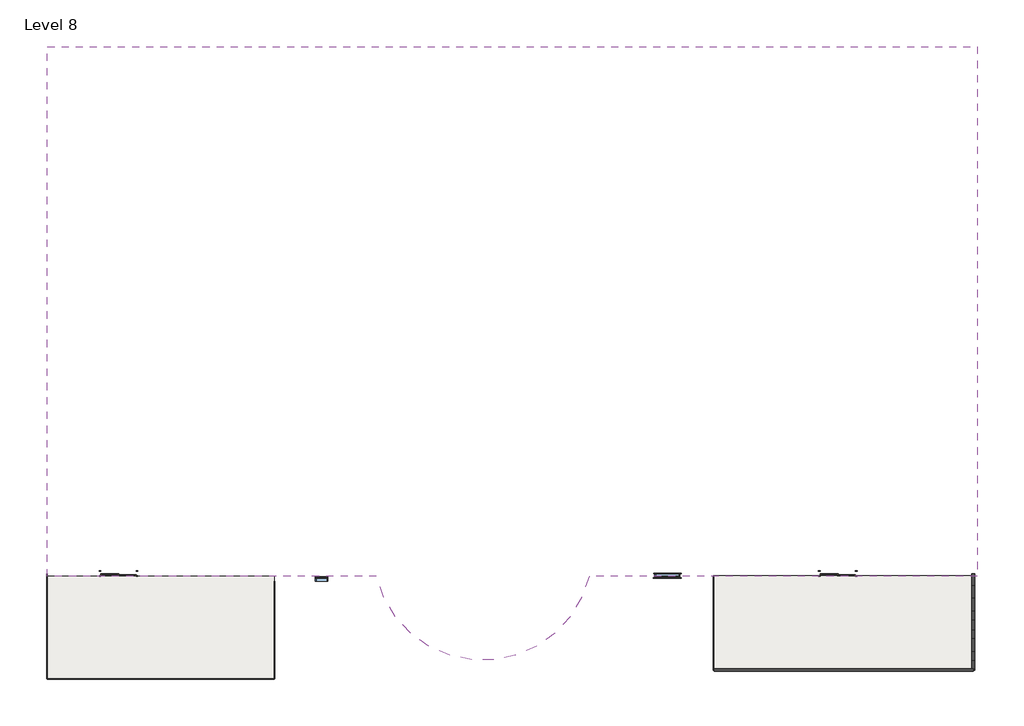
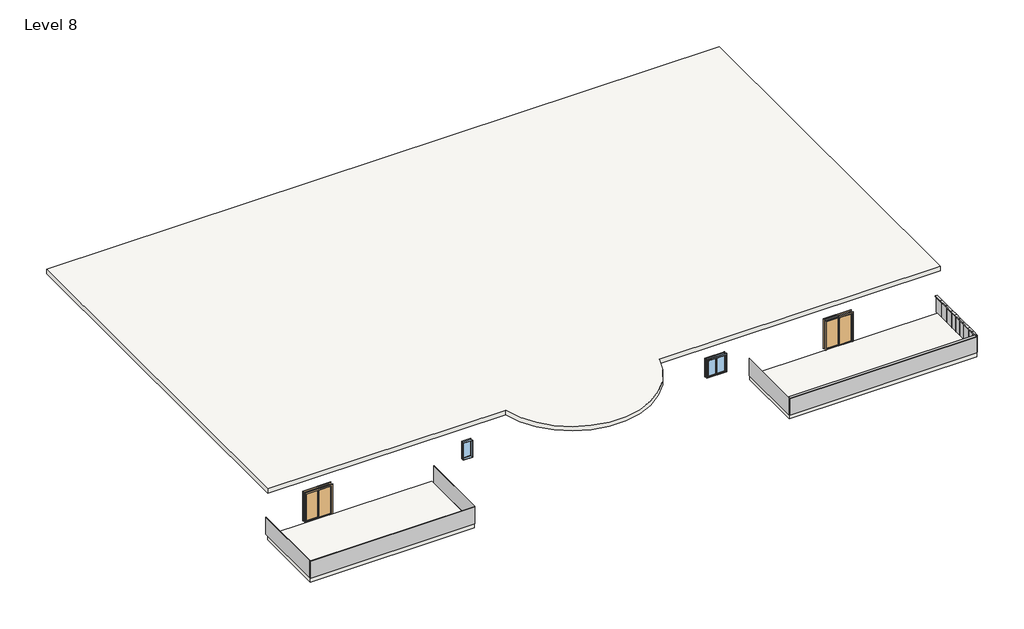
# One storey: 14 plates, 11 members, 3 slabs, 2 doors, 2 windows.
"""IFC4 building model written with IfcOpenShell, lengths in millimetres."""

from ifc_helpers import new_model, si_unit, point, frame, frame_2d, origin, place, context, project, spatial, polyline, circle_curve, trimmed, segment, composite_curve, outline, extrude, transform, mapped, element, save
from components import door_076b30e0, member_47bfaf8a, member_75074519, member_7096a90e, member_15823cb3, member_00d8fd3b, member_943fafd7, system_panel_glazed_2c1c32f8, system_panel_glazed_7af1c9c3, system_panel_glazed_a18a7e0a, system_panel_glazed_c3939aa2, system_panel_glazed_7487696a, system_panel_glazed_8d5a176b, system_panel_glazed_b96adab1, system_panel_glazed_1e6177f2, system_panel_glazed_2980b8bc, window_0862ab64, window_80bd9af0

model = new_model("IFC4")

# Units and contexts
model_context = context("Model", 3, world=origin())
ifc_project = project(units=[si_unit("LENGTHUNIT", "METRE", prefix="MILLI")], contexts=[model_context])

# Site, building, storey
site = spatial("IfcSite", under=ifc_project)
building = spatial("IfcBuilding", under=site)
storey = spatial("IfcBuildingStorey", under=building, Name="Level 8", Elevation=13106.4)

# Doors
placement = place(None, origin())
door_shape = door_076b30e0(model_context)
element("IfcDoor", 1, ObjectType="Door-Double-Sliding : 68\" x 80\"", at=placement, inside=storey, context=model_context, shape_type="MappedRepresentation", body=[
    mapped(door_shape, transform((-16369.385279, -12227.7237084, 13106.4), x_axis=(-1.0, 0.0, 0.0), y_axis=(0.0, -1.0, 0.0), z_axis=(0.0, 0.0, 1.0))),
])
element("IfcDoor", 2, ObjectType="Door-Double-Sliding : 68\" x 80\"", at=placement, inside=storey, context=model_context, shape_type="MappedRepresentation", body=[
    mapped(door_shape, transform((18682.614721, -12227.7237084, 13106.4), x_axis=(-1.0, 0.0, 0.0), y_axis=(0.0, -1.0, 0.0), z_axis=(0.0, 0.0, 1.0))),
])

# Members
member_shape = member_47bfaf8a(model_context)
element("IfcMember", 3, ObjectType="Rectangular Mullion : 2.5\" x 5\" rectangular", at=placement, inside=storey, context=model_context, shape_type="MappedRepresentation", body=[
    mapped(member_shape, transform((25286.614721, -16149.2463689, 14325.6), x_axis=(0.0, 0.0, 1.0), y_axis=(-1.0, 0.0, 0.0), z_axis=(0.0, -1.0, 0.0))),
])
member_2_shape = member_75074519(model_context)
element("IfcMember", 4, ObjectType="Rectangular Mullion : 2.5\" x 5\" rectangular", at=placement, inside=storey, context=model_context, shape_type="MappedRepresentation", body=[
    mapped(member_2_shape, transform((25286.614721, -17063.6463689, 13106.4), x_axis=(0.0, -1.0, 0.0), y_axis=(-1.0, 0.0, 0.0), z_axis=(0.0, 0.0, -1.0))),
])
member_3_shape = member_7096a90e(model_context)
element("IfcMember", 5, ObjectType="Rectangular Mullion : 2.5\" x 5\" rectangular", at=placement, inside=storey, context=model_context, shape_type="MappedRepresentation", body=[
    mapped(member_3_shape, transform((25286.614721, -17000.1463689, 14325.6), x_axis=(0.0, 0.0, 1.0), y_axis=(-1.0, 0.0, 0.0), z_axis=(0.0, -1.0, 0.0))),
])
member_4_shape = member_15823cb3(model_context)
element("IfcMember", 6, ObjectType="Rectangular Mullion : 2.5\" x 5\" rectangular", at=placement, inside=storey, context=model_context, shape_type="MappedRepresentation", body=[
    mapped(member_4_shape, transform((25286.614721, -14625.2463689, 14325.6), x_axis=(0.0, 0.0, 1.0), y_axis=(-1.0, 0.0, 0.0), z_axis=(0.0, -1.0, 0.0))),
])
element("IfcMember", 7, ObjectType="Rectangular Mullion : 2.5\" x 5\" rectangular", at=placement, inside=storey, context=model_context, shape_type="MappedRepresentation", body=[
    mapped(member_4_shape, transform((25286.614721, -15082.4463689, 14325.6), x_axis=(0.0, 0.0, 1.0), y_axis=(-1.0, 0.0, 0.0), z_axis=(0.0, -1.0, 0.0))),
])
element("IfcMember", 8, ObjectType="Rectangular Mullion : 2.5\" x 5\" rectangular", at=placement, inside=storey, context=model_context, shape_type="MappedRepresentation", body=[
    mapped(member_4_shape, transform((25286.614721, -15539.6463689, 14325.6), x_axis=(0.0, 0.0, 1.0), y_axis=(-1.0, 0.0, 0.0), z_axis=(0.0, -1.0, 0.0))),
])
element("IfcMember", 9, ObjectType="Rectangular Mullion : 2.5\" x 5\" rectangular", at=placement, inside=storey, context=model_context, shape_type="MappedRepresentation", body=[
    mapped(member_4_shape, transform((25286.614721, -16606.4463689, 14325.6), x_axis=(0.0, 0.0, 1.0), y_axis=(-1.0, 0.0, 0.0), z_axis=(0.0, -1.0, 0.0))),
])
member_5_shape = member_00d8fd3b(model_context)
element("IfcMember", 10, ObjectType="Rectangular Mullion : 2.5\" x 5\" rectangular", at=placement, inside=storey, context=model_context, shape_type="MappedRepresentation", body=[
    mapped(member_5_shape, transform((25286.614721, -12959.1645952, 14325.6), x_axis=(0.0, 0.0, 1.0), y_axis=(-1.0, 0.0, 0.0), z_axis=(0.0, -1.0, 0.0))),
])
element("IfcMember", 11, ObjectType="Rectangular Mullion : 2.5\" x 5\" rectangular", at=placement, inside=storey, context=model_context, shape_type="MappedRepresentation", body=[
    mapped(member_5_shape, transform((25286.614721, -13563.605482, 14325.6), x_axis=(0.0, 0.0, 1.0), y_axis=(-1.0, 0.0, 0.0), z_axis=(0.0, -1.0, 0.0))),
])
element("IfcMember", 12, ObjectType="Rectangular Mullion : 2.5\" x 5\" rectangular", at=placement, inside=storey, context=model_context, shape_type="MappedRepresentation", body=[
    mapped(member_5_shape, transform((25286.614721, -14168.0463689, 14325.6), x_axis=(0.0, 0.0, 1.0), y_axis=(-1.0, 0.0, 0.0), z_axis=(0.0, -1.0, 0.0))),
])
member_6_shape = member_943fafd7(model_context)
element("IfcMember", 13, ObjectType="Rectangular Mullion : 2.5\" x 5\" rectangular", at=placement, inside=storey, context=model_context, shape_type="MappedRepresentation", body=[
    mapped(member_6_shape, transform((12667.5594464, -17063.6463689, 14325.6), x_axis=(0.0, 0.0, 1.0), y_axis=(0.0, 1.0, 0.0), z_axis=(-1.0, 0.0, 0.0))),
])

# Plates
system_panel_glazed_shape = system_panel_glazed_2c1c32f8(model_context)
element("IfcPlate", 14, ObjectType="System Panel : Glazed", at=placement, inside=storey, context=model_context, shape_type="MappedRepresentation", body=[
    mapped(system_panel_glazed_shape, transform((12667.5594464, -14759.9850386, 13106.4), x_axis=(0.0, 1.0, 0.0), y_axis=(-1.0, 0.0, 0.0), z_axis=(0.0, 0.0, 1.0))),
])
system_panel_glazed_2_shape = system_panel_glazed_7af1c9c3(model_context)
element("IfcPlate", 15, ObjectType="System Panel : Glazed", at=placement, inside=storey, context=model_context, shape_type="MappedRepresentation", body=[
    mapped(system_panel_glazed_2_shape, transform((25286.614721, -15844.4463689, 13106.4), x_axis=(0.0, -1.0, 0.0), y_axis=(1.0, 0.0, 0.0), z_axis=(0.0, 0.0, 1.0))),
])
system_panel_glazed_3_shape = system_panel_glazed_a18a7e0a(model_context)
element("IfcPlate", 16, ObjectType="System Panel : Glazed", at=placement, inside=storey, context=model_context, shape_type="MappedRepresentation", body=[
    mapped(system_panel_glazed_3_shape, transform((25286.614721, -16377.8463689, 13106.4), x_axis=(0.0, -1.0, 0.0), y_axis=(1.0, 0.0, 0.0), z_axis=(0.0, 0.0, 1.0))),
])
element("IfcPlate", 17, ObjectType="System Panel : Glazed", at=placement, inside=storey, context=model_context, shape_type="MappedRepresentation", body=[
    mapped(system_panel_glazed_3_shape, transform((25286.614721, -15311.0463689, 13106.4), x_axis=(0.0, -1.0, 0.0), y_axis=(1.0, 0.0, 0.0), z_axis=(0.0, 0.0, 1.0))),
])
element("IfcPlate", 18, ObjectType="System Panel : Glazed", at=placement, inside=storey, context=model_context, shape_type="MappedRepresentation", body=[
    mapped(system_panel_glazed_3_shape, transform((25286.614721, -14853.8463689, 13106.4), x_axis=(0.0, -1.0, 0.0), y_axis=(1.0, 0.0, 0.0), z_axis=(0.0, 0.0, 1.0))),
])
element("IfcPlate", 19, ObjectType="System Panel : Glazed", at=placement, inside=storey, context=model_context, shape_type="MappedRepresentation", body=[
    mapped(system_panel_glazed_3_shape, transform((25286.614721, -14396.6463689, 13106.4), x_axis=(0.0, -1.0, 0.0), y_axis=(1.0, 0.0, 0.0), z_axis=(0.0, 0.0, 1.0))),
])
system_panel_glazed_4_shape = system_panel_glazed_c3939aa2(model_context)
element("IfcPlate", 20, ObjectType="System Panel : Glazed", at=placement, inside=storey, context=model_context, shape_type="MappedRepresentation", body=[
    mapped(system_panel_glazed_4_shape, transform((25286.614721, -16803.2963689, 13106.4), x_axis=(0.0, -1.0, 0.0), y_axis=(1.0, 0.0, 0.0), z_axis=(0.0, 0.0, 1.0))),
])
system_panel_glazed_5_shape = system_panel_glazed_7487696a(model_context)
element("IfcPlate", 21, ObjectType="System Panel : Glazed", at=placement, inside=storey, context=model_context, shape_type="MappedRepresentation", body=[
    mapped(system_panel_glazed_5_shape, transform((25286.614721, -12656.9441518, 13106.4), x_axis=(0.0, -1.0, 0.0), y_axis=(1.0, 0.0, 0.0), z_axis=(0.0, 0.0, 1.0))),
])
element("IfcPlate", 22, ObjectType="System Panel : Glazed", at=placement, inside=storey, context=model_context, shape_type="MappedRepresentation", body=[
    mapped(system_panel_glazed_5_shape, transform((25286.614721, -13865.8259254, 13106.4), x_axis=(0.0, -1.0, 0.0), y_axis=(1.0, 0.0, 0.0), z_axis=(0.0, 0.0, 1.0))),
])
element("IfcPlate", 23, ObjectType="System Panel : Glazed", at=placement, inside=storey, context=model_context, shape_type="MappedRepresentation", body=[
    mapped(system_panel_glazed_5_shape, transform((25286.614721, -13261.3850386, 13106.4), x_axis=(0.0, -1.0, 0.0), y_axis=(1.0, 0.0, 0.0), z_axis=(0.0, 0.0, 1.0))),
])
system_panel_glazed_6_shape = system_panel_glazed_8d5a176b(model_context)
element("IfcPlate", 24, ObjectType="System Panel : Glazed", at=placement, inside=storey, context=model_context, shape_type="MappedRepresentation", body=[
    mapped(system_panel_glazed_6_shape, transform((18977.0870837, -17063.6463689, 13106.4), x_axis=(-1.0, 0.0, 0.0), y_axis=(0.0, -1.0, 0.0), z_axis=(0.0, 0.0, 1.0))),
])
system_panel_glazed_7_shape = system_panel_glazed_b96adab1(model_context)
element("IfcPlate", 25, ObjectType="System Panel : Glazed", at=placement, inside=storey, context=model_context, shape_type="MappedRepresentation", body=[
    mapped(system_panel_glazed_7_shape, transform((-14302.7926538, -17468.9486425, 13106.4), x_axis=(-1.0, 0.0, 0.0), y_axis=(0.0, -1.0, 0.0), z_axis=(0.0, 0.0, 1.0))),
])
system_panel_glazed_8_shape = system_panel_glazed_1e6177f2(model_context)
element("IfcPlate", 26, ObjectType="System Panel : Glazed", at=placement, inside=storey, context=model_context, shape_type="MappedRepresentation", body=[
    mapped(system_panel_glazed_8_shape, transform((-19823.785279, -14911.8361754, 13106.4), x_axis=(0.0, 1.0, 0.0), y_axis=(-1.0, 0.0, 0.0), z_axis=(0.0, 0.0, 1.0))),
])
system_panel_glazed_9_shape = system_panel_glazed_2980b8bc(model_context)
element("IfcPlate", 27, ObjectType="System Panel : Glazed", at=placement, inside=storey, context=model_context, shape_type="MappedRepresentation", body=[
    mapped(system_panel_glazed_9_shape, transform((-8781.8000285, -15093.8746867, 13106.4), x_axis=(0.0, -1.0, 0.0), y_axis=(1.0, 0.0, 0.0), z_axis=(0.0, 0.0, 1.0))),
])

# Slabs
element("IfcSlab", 28, ObjectType="Generic - 12\"", at=placement, inside=storey, context=model_context, shape_type="SweptSolid", body=[
    extrude(outline(composite_curve([segment(polyline([(25489.814721, 13322.6839017), (25489.814721, -12483.7160983), (6571.5594464, -12483.7160983)]), True, "CONTINUOUS"), segment(trimmed(circle_curve(frame_2d((1385.214721, -11253.083057)), 5330.3498284), [point((6571.5594464, -12483.7160983))], [point((-3801.1300045, -12483.7160983))], False, "CARTESIAN"), True, "CONTINUOUS"), segment(polyline([(-3801.1300045, -12483.7160983), (-19823.785279, -12483.7160983), (-19823.785279, 13322.6839017), (25489.814721, 13322.6839017)]), True, "CONTINUOUS")], self_intersect=False)), frame((0.0, 0.0, 16103.4634343), z_axis=(0.0, 0.0, 1.0), x_axis=(1.0, 0.0, 0.0)), (0.0, 0.0, 1.0), 304.8),
])
element("IfcSlab", 29, ObjectType="Generic - 12\"", at=placement, inside=storey, context=model_context, shape_type="SweptSolid", body=[
    extrude(outline(polyline([(25286.614721, -12456.3237084), (25286.614721, -17063.6463689), (12667.5594464, -17063.6463689), (12667.5594464, -12456.3237084), (25286.614721, -12456.3237084)])), frame((0.0, 0.0, 12801.6), z_axis=(0.0, 0.0, 1.0), x_axis=(1.0, 0.0, 0.0)), (0.0, 0.0, 1.0), 304.8),
])
element("IfcSlab", 30, ObjectType="Generic - 12\"", at=placement, inside=storey, context=model_context, shape_type="SweptSolid", body=[
    extrude(outline(polyline([(-8781.8000285, -12483.7160983), (-8781.8000285, -17468.9486425), (-19823.785279, -17468.9486425), (-19823.785279, -12483.7160983), (-8781.8000285, -12483.7160983)])), frame((0.0, 0.0, 12801.6), z_axis=(0.0, 0.0, 1.0), x_axis=(1.0, 0.0, 0.0)), (0.0, 0.0, 1.0), 304.8),
])

# Windows
window_shape = window_0862ab64(model_context)
element("IfcWindow", 31, ObjectType="Casement Dbl with Trim : 48\" x 48\"", at=placement, inside=storey, context=model_context, shape_type="MappedRepresentation", body=[
    mapped(window_shape, transform((10381.5594464, -12437.2737084, 13106.4), x_axis=(-1.0, 0.0, 0.0), y_axis=(0.0, -1.0, 0.0), z_axis=(0.0, 0.0, 1.0))),
])
window_2_shape = window_80bd9af0(model_context)
element("IfcWindow", 32, ObjectType="Fixed : 24\" x 48\"", at=placement, inside=storey, context=model_context, shape_type="MappedRepresentation", body=[
    mapped(window_2_shape, transform((-6425.285279, -12617.2007309, 13106.4), x_axis=(1.0, 0.0, 0.0), y_axis=(0.0, 1.0, 0.0), z_axis=(0.0, 0.0, 1.0))),
])

save(model, "model.ifc")

# Revit data of these elements
# Type "Door-Double-Sliding : 68\" x 80\""
#   Type Mark = "10"
#   Construction Type Id = "opn-d45"
#   Assembly Code = "C1020"
#   Analytic Construction = "Wood frame, double glass door "
#   Thickness = 0' - 2"
#   Thermal Resistance (R) = 1.8150 (h·ft²·°F)/BTU
#   Heat Transfer Coefficient (U) = 0.5510 BTU/(h·ft²·°F)
#   Height = 6' - 8"
#   Rail Width = 0' - 2"
#   Stiles = 0' - 2"
#   Trim Projection Ext = 0' - 1"
#   Trim Projection Int = 0' - 1"
#   Trim Width = 0' - 3"
#   Width = 5' - 8"
#   Define Thermal Properties by = 1
#   Glazing = Glass
#   Panel Material = Wood - Birch - Solid Stained Light Low Gloss
#   Trim Material = Paint - Sienna
#   Visual Light Transmittance = 0
#   Solar Heat Gain Coefficient = 0
#   Function = (empty or 0)
#   Wall Closure = (empty or 0)
# Type "Rectangular Mullion : 2.5\" x 5\" rectangular"
#   built-in parameter 1007304 = 0.416667 (stored number, unit not read)
#   built-in parameter 1007301 = 0.104167 (stored number, unit not read)
#   built-in parameter 1007300 = 0.104167 (stored number, unit not read)
# Type "System Panel : Glazed"
#   Construction Type Id = "GSP4R"
#   Analytic Construction = "1/8 in Pilkington single glazing"
#   Visual Light Transmittance = 0.9
#   Solar Heat Gain Coefficient = 0.86
#   Heat Transfer Coefficient (U) = 1.18115 BTU/(h·ft²·°F)
# Type "Generic - 12\""
#   Assembly Code = "B1010"
#   Function = 0
#   Layers, outside or top first: 1' - 0" no material (function 1)
# Type "Casement Dbl with Trim : 48\" x 48\""
#   Type Mark = "34"
#   Construction Type Id = "GSP4R"
#   Assembly Code = "B2020100"
#   Analytic Construction = "1/8 in Pilkington single glazing"
#   Visual Light Transmittance = 0.9
#   Solar Heat Gain Coefficient = 0.78
#   Heat Transfer Coefficient (U) = 0.6496 BTU/(h·ft²·°F)
#   Height = 4' - 0"
#   Default Sill Height = 3' - 0"
#   Trim Projection - Ext. = 0' - 0 1/2"
#   Trim Projection - Int. = 0' - 0 3/4"
#   Trim Width - Exterior = 0' - 3 1/2"
#   Trim Width - Interior = 0' - 3 1/2"
#   Width = 4' - 0"
#   Window Inset = 0' - 0 3/4"
#   Define Thermal Properties by = 1
#   Glass Pane Material = Glass
#   Sash Material = Sash
#   Trim Exterior Material = Trim
#   Trim Interior Material = Trim
#   Wall Closure = (empty or 0)
# Type "Fixed : 24\" x 48\""
#   Type Mark = "2"
#   Construction Type Id = "GSP4R"
#   Assembly Code = "B2020100"
#   Analytic Construction = "1/8 in Pilkington single glazing"
#   Visual Light Transmittance = 0.9
#   Solar Heat Gain Coefficient = 0.78
#   Heat Transfer Coefficient (U) = 0.6496 BTU/(h·ft²·°F)
#   Height = 4' - 0"
#   Default Sill Height = 3' - 0"
#   Width = 2' - 0"
#   Window Inset = 0' - 0 3/4"
#   Define Thermal Properties by = 1
#   Glass Pane Material = Glass
#   Sash Material = Sash
#   Wall Closure = (empty or 0)
# Elements 1, 2 (IfcDoor, "Door-Double-Sliding : 68\" x 80\"")
#   Phase Created = New Construction
#   Materials on its faces: "Paint - Sienna", "Wood - Birch - Solid Stained Light Low Gloss", "Glass"
# Elements 3, 4, 5, 6, 7, 8, 9, 10, 11, 12, 13 (IfcMember, "Rectangular Mullion : 2.5\" x 5\" rectangular")
#   Phase Created = New Construction
#   Materials on its faces: "Aluminum"
# Elements 14, 15, 16, 17, 18, 19, 20, 21, 22, 23, 24, 25, 26, 27 (IfcPlate, "System Panel : Glazed")
#   Phase Created = New Construction
#   Materials on its faces: "Glass"
# Element 28 (IfcSlab, "Generic - 12\"")
#   Height Offset From Level = 10' - 9.99462"
#   Phase Created = New Construction
#   Materials on its faces: "Default Floor"
# Elements 29, 30 (IfcSlab, "Generic - 12\"")
#   Height Offset From Level = 0' - 0"
#   Phase Created = New Construction
#   Materials on its faces: "Default Floor"
# Element 31 (IfcWindow, "Casement Dbl with Trim : 48\" x 48\"")
#   Mark = "13"
#   Phase Created = New Construction
#   Materials on its faces: "Sash", "Trim", "Glass"
# Element 32 (IfcWindow, "Fixed : 24\" x 48\"")
#   Mark = "81"
#   Phase Created = New Construction
#   Materials on its faces: "Sash", "Glass"
# Materials
#   "Glass": class "Glass", colour RGB 0 128 192, transparency 0.75, Description = "Soda Lime Glass", Cost = 0
#   "Wood - Birch - Solid Stained Light Low Gloss": class "Wood", colour RGB 210 159 95, transparency 0, Cost = 0
#   "Paint - Sienna": colour RGB 118 70 51, transparency 0, Cost = 0
#   "Sash": class "Wood", colour RGB 224 178 126, transparency 0
#   "Trim": class "Wood", colour RGB 224 178 126, transparency 0
#   "Aluminum": class "Metal", colour RGB 247 247 247, transparency 0, Description = "Aluminum 6061", Cost = 0
#   "Default Floor": colour RGB 128 128 128, transparency 0
